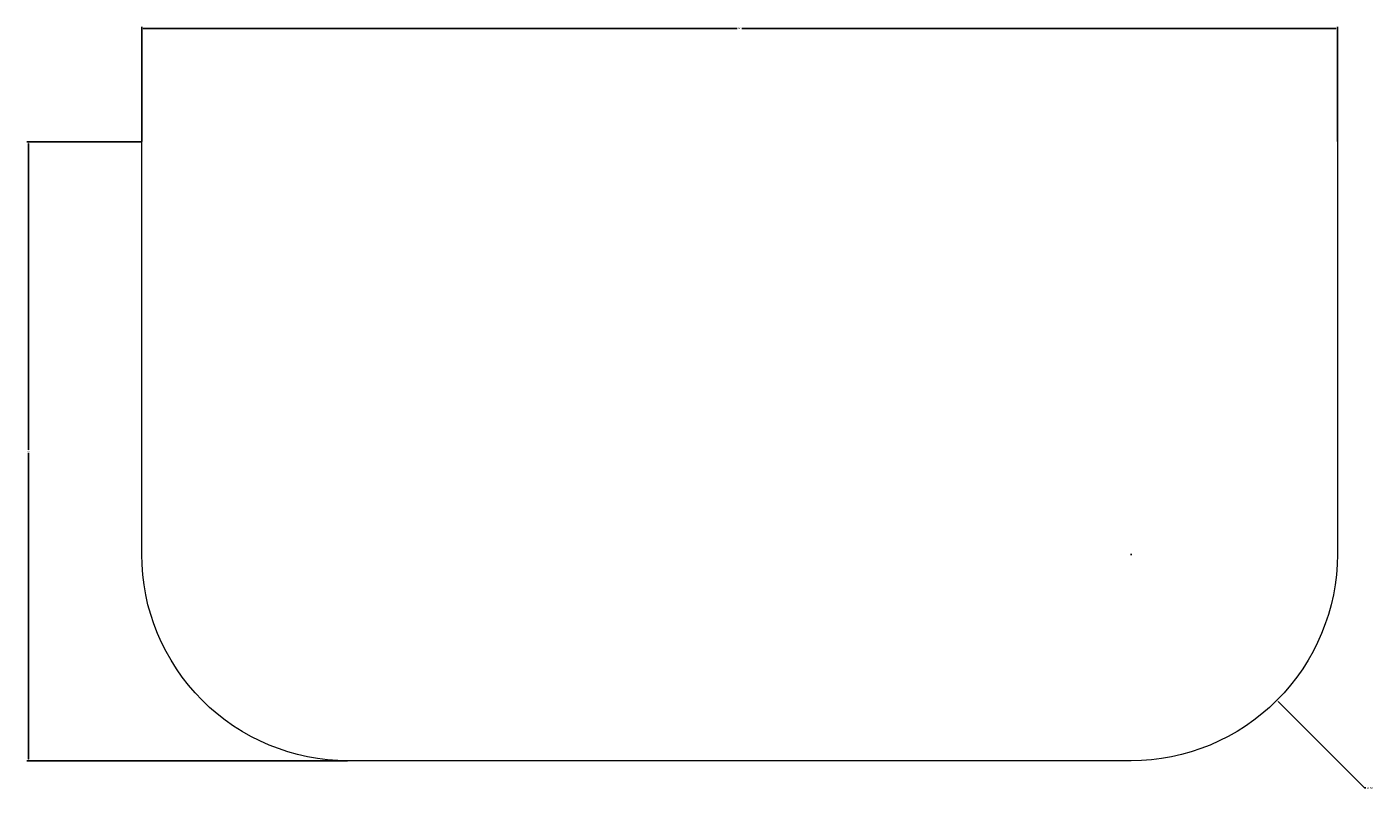
# Model space of a CAD drawing. Units: millimetres. Extents: x 210 to 373, y 840 to 932.
import ezdxf

# ---------------------------------------------------------------- set-up
doc = ezdxf.new("R2010")
doc.units = ezdxf.units.MM
doc.layers.add('M-CONS', color=8, linetype='Continuous', lineweight=18)
doc.layers.add('M-DIMS', color=2, linetype='Continuous', lineweight=18)
doc.styles.get("Standard").update_dxf_attribs({"font": 'arial.ttf'})
doc.dimstyles.get("Standard").update_dxf_attribs({"dimtxt": 0.18, "dimasz": 0.18, "dimexe": 0.18, "dimexo": 0.0625, "dimgap": 0.09, "dimtad": 0, "dimtih": 1, "dimtoh": 1, "dimdec": 4, "dimzin": 0, "dimdsep": 46, "dimtxsty": 'Standard', "dimcen": 0.09, "dimadec": 0, "dimazin": 0, "dimtfac": 1, "dimtdec": 4, "dimtofl": 0, "dimtmove": 0, "dimatfit": 3, "dimfxl": 1, "dimtolj": 1, "dimtzin": 0, "dimarcsym": 0})

# ---------------------------------------------------------------- blocks, each defined once
blk = doc.blocks.new('*D1')
at = {"layer": 'Defpoints', "color": 0, "transparency": 16777216}
for p in [(368.5, 931.86), (223.5, 918.11), (368.5, 918.11)]:
    blk.add_point(p, dxfattribs=at)
at = {"layer": 'M-DIMS', "color": 0, "lineweight": -2, "transparency": 16777216}
for p, q in [((223.5, 918.17), (223.5, 932.04)), ((223.68, 931.86), (295.72, 931.86)), ((368.32, 931.86), (296.28, 931.86)), ((368.5, 918.17), (368.5, 932.04))]:
    blk.add_line(p, q, dxfattribs=at)
at = {"layer": 'M-DIMS', "color": 0, "transparency": 16777216}
for points in [[(223.68, 931.89), (223.68, 931.83), (223.5, 931.86)], [(368.32, 931.89), (368.32, 931.83), (368.5, 931.86)]]:
    blk.add_solid(points, dxfattribs=at)
at = {"layer": 'M-DIMS', "color": 0, "transparency": 16777216, "insert": (296, 931.86), "char_height": 0.18, "attachment_point": 5}
blk.add_mtext('\\A1;145', dxfattribs=at)
blk = doc.blocks.new('*D2')
at = {"layer": 'Defpoints', "color": 0, "transparency": 16777216}
for p in [(209.75, 918.11), (223.5, 918.11), (248.5, 843.11)]:
    blk.add_point(p, dxfattribs=at)
at = {"layer": 'M-DIMS', "color": 0, "lineweight": -2, "transparency": 16777216}
for p, q in [((223.44, 918.11), (209.57, 918.11)), ((209.75, 917.93), (209.75, 880.79)), ((209.75, 843.29), (209.75, 880.42)), ((248.44, 843.11), (209.57, 843.11))]:
    blk.add_line(p, q, dxfattribs=at)
at = {"layer": 'M-DIMS', "color": 0, "transparency": 16777216}
for points in [[(209.72, 917.93), (209.78, 917.93), (209.75, 918.11)], [(209.72, 843.29), (209.78, 843.29), (209.75, 843.11)]]:
    blk.add_solid(points, dxfattribs=at)
at = {"layer": 'M-DIMS', "color": 0, "transparency": 16777216, "insert": (209.75, 880.61), "char_height": 0.18, "attachment_point": 5}
blk.add_mtext('\\A1;75', dxfattribs=at)
blk = doc.blocks.new('*D3')
at = {"layer": 'Defpoints', "color": 0, "transparency": 16777216}
for p in [(343.5, 868.11), (361.18, 850.43)]:
    blk.add_point(p, dxfattribs=at)
at = {"layer": 'M-DIMS', "color": 0, "lineweight": -2, "transparency": 16777216}
for p, q in [((343.41, 868.11), (343.59, 868.11)), ((343.5, 868.02), (343.5, 868.2)), ((371.79, 839.82), (361.31, 850.3)), ((371.97, 839.82), (371.79, 839.82))]:
    blk.add_line(p, q, dxfattribs=at)
at = {"layer": 'M-DIMS', "color": 0, "transparency": 16777216}
blk.add_solid([(361.33, 850.32), (361.29, 850.28), (361.18, 850.43)], dxfattribs=at)
at = {"layer": 'M-DIMS', "color": 0, "transparency": 16777216, "insert": (372.47, 839.82), "char_height": 0.18, "attachment_point": 5}
blk.add_mtext('\\A1;2X R25', dxfattribs=at)

msp = doc.modelspace()

# ---------------------------------------------------------------- linework, layer by layer
at = {"layer": 'M-CONS', "elevation": 12}
msp.add_lwpolyline([(368.5, 918.11), (368.5, 868.11, -0.414214), (343.5, 843.11), (248.5, 843.11, -0.414214), (223.5, 868.11), (223.5, 918.11)], format="xyb", dxfattribs=at)

# ---------------------------------------------------------------- dimensions: what is measured, and where the dimension line sits
at = {"layer": 'M-DIMS'}
dim = msp.add_linear_dim(base=(368.5, 931.86), p1=(223.5, 918.11), p2=(368.5, 918.11), dimstyle='Standard', override={"dimdec": 0, "dimlfac": 1, "dimrnd": 0, "dimzin": 0, "dimdsep": 46, "dimlunit": 2}, dxfattribs=at)
dim.commit()
dim.dimension.update_dxf_attribs({"geometry": '*D1', "text_midpoint": (296, 931.86)})
dim = msp.add_linear_dim(base=(209.75, 918.11), p1=(248.5, 843.11), p2=(223.5, 918.11), angle=90, dimstyle='Standard', override={"dimdec": 0, "dimlfac": 1, "dimrnd": 0, "dimzin": 0, "dimdsep": 46, "dimlunit": 2}, dxfattribs=at)
dim.commit()
dim.dimension.update_dxf_attribs({"geometry": '*D2', "text_midpoint": (209.75, 880.61)})
dim = msp.add_radius_dim(center=(343.5, 868.11), mpoint=(361.18, 850.43), text='2X <>', dimstyle='Standard', override={"dimdec": 0, "dimlfac": 1, "dimrnd": 0, "dimzin": 0, "dimdsep": 46, "dimlunit": 2}, dxfattribs=at)
dim.commit()
dim.dimension.update_dxf_attribs({"geometry": '*D3', "text_midpoint": (372.47, 839.82), "dimtype": 164})

doc.saveas('drawing.dxf')
